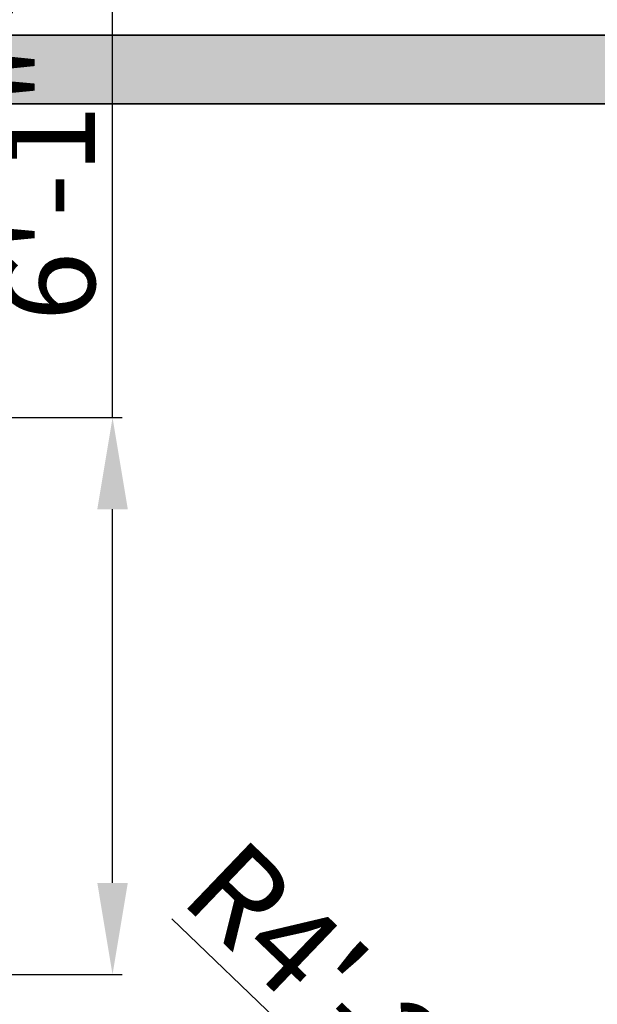
# Model space of a CAD drawing. Units: inches. Extents: x 2083 to 3317, y 1141 to 2115.
# Tile 100 of 256: x 2339 to 2415, y 1894 to 2023. Entities that reach past the tile are written whole.
import ezdxf

# ---------------------------------------------------------------- set-up
doc = ezdxf.new("R2010")
doc.units = ezdxf.units.IN
doc.layers.add('A-ANNO-DIMS', color=2, linetype='Continuous', lineweight=18)
doc.layers.add('A-WALL', color=7, linetype='Continuous', lineweight=35)
doc.layers.add('A-WALL-PATT', color=251, linetype='Continuous', lineweight=13, true_color=0x636466)
doc.styles.get("Standard").update_dxf_attribs({"font": 'arial.ttf'})
doc.dimstyles.new('ISO-25', dxfattribs={"dimtxt": 12, "dimasz": 12, "dimexe": 1.25, "dimexo": 0.625, "dimtad": 1, "dimlunit": 3, "dimtxsty": 'Standard', "dimcen": 2.5, "dimadec": 0, "dimazin": 0, "dimtfac": 1, "dimtmove": 0, "dimatfit": 3, "dimfxl": 1, "dimarcsym": 0})

# ---------------------------------------------------------------- blocks, each defined once
blk = doc.blocks.new('*D21')
at = {"layer": 'A-ANNO-DIMS', "color": 0, "lineweight": -2, "transparency": 16777216}
for p, q in [((2351.18, 1970.69), (2351.18, 2057.15)), ((2337.85, 1970.69), (2352.43, 1970.69)), ((2351.18, 1909.74), (2351.18, 1958.69)), ((2337.85, 1897.74), (2352.43, 1897.74))]:
    blk.add_line(p, q, dxfattribs=at)
at = {"layer": 'A-ANNO-DIMS', "color": 0, "transparency": 16777216}
for points in [[(2349.18, 1958.69), (2353.18, 1958.69), (2351.18, 1970.69)], [(2349.18, 1909.74), (2353.18, 1909.74), (2351.18, 1897.74)]]:
    blk.add_solid(points, dxfattribs=at)
at = {"layer": 'Defpoints', "color": 0, "transparency": 16777216}
for p in [(2337.22, 1970.69), (2351.18, 1970.69), (2337.22, 1897.74)]:
    blk.add_point(p, dxfattribs=at)
at = {"layer": 'A-ANNO-DIMS', "color": 0, "transparency": 16777216, "insert": (2344.43, 2019.92), "char_height": 12, "attachment_point": 5, "rotation": 90}
blk.add_mtext('6\'-1" TYP.', dxfattribs=at)
blk = doc.blocks.new('*D36')
at = {"layer": 'A-ANNO-DIMS', "color": 0, "lineweight": -2, "transparency": 16777216}
for p, q in [((2235.96, 2012.39), (2235.96, 2074.36)), ((2471.46, 2012.39), (2471.46, 2074.36)), ((2247.96, 2073.11), (2459.46, 2073.11))]:
    blk.add_line(p, q, dxfattribs=at)
at = {"layer": 'A-ANNO-DIMS', "color": 0, "transparency": 16777216}
for points in [[(2247.96, 2075.11), (2247.96, 2071.11), (2235.96, 2073.11)], [(2459.46, 2075.11), (2459.46, 2071.11), (2471.46, 2073.11)]]:
    blk.add_solid(points, dxfattribs=at)
at = {"layer": 'Defpoints', "color": 0, "transparency": 16777216}
for p in [(2471.46, 2073.11), (2235.96, 2011.76), (2471.46, 2011.76)]:
    blk.add_point(p, dxfattribs=at)
at = {"layer": 'A-ANNO-DIMS', "color": 0, "transparency": 16777216, "insert": (2353.71, 2079.94), "char_height": 12, "attachment_point": 5}
blk.add_mtext('19\'-7 1/2"', dxfattribs=at)
blk = doc.blocks.new('*D68')
at = {"layer": 'A-ANNO-DIMS', "color": 0, "lineweight": -2, "transparency": 16777216}
for p, q in [((2358.93, 1905.02), (2420.01, 1846.48)), ((2465.03, 1803.34), (2428.67, 1838.18))]:
    blk.add_line(p, q, dxfattribs=at)
at = {"layer": 'A-ANNO-DIMS', "color": 0, "transparency": 16777216}
blk.add_solid([(2421.39, 1847.93), (2418.62, 1845.04), (2428.67, 1838.18)], dxfattribs=at)
at = {"layer": 'Defpoints', "color": 0, "transparency": 16777216}
for p in [(2428.67, 1838.18), (2465.03, 1803.34)]:
    blk.add_point(p, dxfattribs=at)
at = {"layer": 'A-ANNO-DIMS', "color": 0, "transparency": 16777216, "insert": (2389.86, 1884.83), "char_height": 12, "attachment_point": 5, "rotation": 316.2184}
blk.add_mtext('R4\'-2 1/2"', dxfattribs=at)

msp = doc.modelspace()

# ---------------------------------------------------------------- hatches: boundary and pattern name
at = {"layer": 'A-WALL-PATT'}
h = msp.add_hatch(color=256, dxfattribs=at)
h.dxf.hatch_style = 1
h.paths.add_polyline_path([(3126.96, 2020.761), (2748.96, 2020.761), (2604.96, 2020.761), (2226.96, 2020.761), (2226.96, 1702.761), (2466.96, 1702.761), (2466.96, 1582.761), (2418.96, 1582.761), (2418.96, 1477.761), (2226.96, 1477.761), (2226.96, 1263.261), (2544.96, 1263.261), (2544.96, 1411.761), (2604.96, 1411.761), (2685.96, 1411.761), (2685.96, 1420.761), (2604.96, 1420.761), (2604.96, 1573.761), (2604.96, 1702.761), (2604.96, 2011.761), (2748.96, 2011.761), (2748.96, 1702.761), (2862.96, 1702.761), (2862.96, 1621.761), (2871.96, 1621.761), (2871.96, 1702.761), (2883.96, 1702.761), (2883.96, 1706.939, -0.0264593), (2883.96, 1711.761), (2757.96, 1711.761), (2757.96, 1807.761), (2787.96, 1807.761), (2787.96, 1812.261), (2757.96, 1812.261), (2757.96, 2011.761), (2877.96, 2011.761), (2877.96, 1812.261), (2847.96, 1812.261), (2847.96, 1807.761), (2889.836, 1807.761), (2889.836, 1812.261), (2882.46, 1812.261), (2882.46, 2011.761), (3117.96, 2011.761), (3117.96, 1812.261), (2937.836, 1812.261), (2937.836, 1807.761), (2995.71, 1807.761), (2995.71, 1796.118), (3000.21, 1796.118), (3000.21, 1807.761), (3117.96, 1807.761), (3117.96, 1711.761), (3000.21, 1711.761), (3000.21, 1760.118), (2998.573, 1760.118, -0.020711), (2995.71, 1760.118), (2995.71, 1711.761), (2931.96, 1711.761), (2931.96, 1702.761), (3126.96, 1702.761)])
h.paths.add_polyline_path([(2471.46, 2011.761), (2471.46, 1810.011), (2462.717, 1810.011), (2462.717, 1805.511), (2505.96, 1805.511), (2505.96, 1810.011), (2475.96, 1810.011), (2475.96, 2011.761), (2595.96, 2011.761), (2595.96, 1810.011), (2565.96, 1810.011), (2565.96, 1805.511), (2595.96, 1805.511), (2595.96, 1711.761), (2235.96, 1711.761), (2235.96, 1805.511), (2353.71, 1805.511), (2353.71, 1796.054), (2358.21, 1796.054), (2358.21, 1805.511), (2414.717, 1805.511), (2414.717, 1810.011), (2235.96, 1810.011), (2235.96, 2011.761)], flags=16)
h.paths.add_polyline_path([(2270.205, 1994.61), (2270.205, 1970.61), (2246.205, 1970.61), (2246.205, 1994.61)], flags=0)
edge = h.paths.add_edge_path(flags=0)
edge.add_ellipse((2332.027, 1899.798), major_axis=(-3.043, 3.043), ratio=0.1682525, start_angle=-161.33217, end_angle=-156.30711, ccw=False)
edge.add_ellipse((2333.082, 1898.744), major_axis=(-1.055, 1.055), ratio=0.4535321, start_angle=-123.37102, end_angle=-94.15911)
edge = h.paths.add_edge_path(flags=0)
edge.add_ellipse((2332.027, 1968.876), major_axis=(3.043, 3.043), ratio=0.1682525, start_angle=18.66783, end_angle=23.69289)
edge.add_spline(control_points=[(2332.926, 1970.691), (2332.227, 1970.336), (2330.894, 1969.659), (2328.413, 1970.932), (2327.204, 1967.749), (2324.71, 1969.956), (2322.533, 1967.012), (2320.013, 1971.296), (2317.68, 1968.158), (2316.041, 1967.102), (2315.427, 1966.81)], knot_values=[0, 0, 0, 0, 2.2670587, 4.3245589, 6.6855835, 8.8786411, 11.121502, 14.300359, 17.7552837, 19.732645, 19.732645, 19.732645, 19.732645], degree=3, periodic=0)
edge.add_ellipse((2332.027, 1968.876), major_axis=(3.043, 3.043), ratio=0.1682525, start_angle=18.66783, end_angle=23.69289, ccw=False)
edge.add_ellipse((2333.082, 1969.931), major_axis=(1.055, 1.055), ratio=0.4535321, start_angle=56.62898, end_angle=85.84089, ccw=False)
edge = h.paths.add_edge_path(flags=0)
edge.add_spline(control_points=[(2296.428, 1967.988), (2293.628, 1965.336), (2287.704, 1959.727), (2299.744, 1949.996), (2294.533, 1935.669), (2290.573, 1920.604), (2293.394, 1909.974), (2296.185, 1904.967)], knot_values=[0.0991853, 0.0991853, 0.0991853, 0.0991853, 0.3453009, 0.6198217, 0.9826526, 1.3860932, 1.8105546, 1.8105546, 1.8105546, 1.8105546], degree=3, periodic=0)
edge.add_spline(control_points=[(2296.185, 1904.967), (2297.384, 1902.619), (2298.001, 1901.949), (2298.553, 1901.468)], knot_values=[0.0062457, 0.0062457, 0.0062457, 0.0062457, 0.0554759, 0.0554759, 0.0554759, 0.0554759], degree=3, periodic=0)
edge.add_spline(control_points=[(2298.553, 1901.468), (2297.259, 1900.923), (2295.225, 1900.232), (2293.06, 1900.614), (2292.101, 1900.788), (2292.09, 1900.791)], knot_values=[0.3128349, 0.3128349, 0.3128349, 0.3128349, 0.4017797, 0.4749867, 0.4759027, 0.4759027, 0.4759027, 0.4759027], degree=3, periodic=0)
edge.add_arc((2292.794, 1904.664), 3.937, 215.4209, 259.69818, ccw=False)
edge.add_spline(control_points=[(2289.585, 1902.382), (2289.477, 1902.535), (2289.368, 1902.688), (2289.261, 1902.841)], knot_values=[0.1028719, 0.1028719, 0.1028719, 0.1028719, 0.1168958, 0.1168958, 0.1168958, 0.1168958], degree=3, periodic=0)
edge.add_spline(control_points=[(2289.261, 1902.841), (2288.687, 1902.55), (2287.64, 1902.02), (2285.881, 1901.874), (2283.853, 1901.504), (2281.72, 1899.711), (2278.467, 1899.493), (2276.157, 1901.883), (2272.259, 1899.804), (2267.778, 1901.843), (2262.244, 1900.184), (2257.415, 1901.782), (2254.318, 1900.726), (2253.178, 1900.337)], knot_values=[0, 0, 0, 0, 1.9079767, 3.4771759, 5.261074, 7.9728515, 11.6802485, 13.7179214, 16.9395917, 22.789562, 27.5025027, 33.5952153, 37.1456181, 37.1456181, 37.1456181, 37.1456181], degree=3, periodic=0)
edge.add_line((2253.178, 1900.337), (2250.244, 1902.841))
edge.add_line((2250.244, 1902.841), (2250.244, 1965.833))
edge.add_line((2250.244, 1965.833), (2253.178, 1968.337))
edge.add_spline(control_points=[(2253.178, 1968.337), (2254.318, 1967.948), (2257.415, 1966.892), (2262.244, 1968.49), (2267.778, 1966.831), (2271.527, 1968.537), (2273.876, 1967.828), (2274.207, 1967.728)], knot_values=[0, 0, 0, 0, 0.0901802, 0.2449351, 0.3646438, 0.5132331, 0.5378548, 0.5378548, 0.5378548, 0.5378548], degree=3, periodic=0)
edge.add_arc((2274.353, 1963.793), 3.937, 72.05113, 92.12795, ccw=False)
edge.add_arc((2281.297, 1985.23), 18.596, 252.05113, 288.56572)
edge.add_arc((2292.317, 1956.029), 12.646, 71.02679, 113.77822, ccw=False)
edge = h.paths.add_edge_path(flags=0)
edge.add_spline(control_points=[(2274.899, 1951.856), (2275.066, 1951.617), (2275.233, 1951.377), (2275.398, 1951.136)], knot_values=[1.4099157, 1.4099157, 1.4099157, 1.4099157, 1.4315903, 1.4315903, 1.4315903, 1.4315903], degree=3, periodic=0)
edge.add_spline(control_points=[(2275.398, 1951.136), (2275.792, 1950.562), (2276.179, 1949.984), (2276.546, 1949.397)], knot_values=[1.3582378, 1.3582378, 1.3582378, 1.3582378, 1.4099157, 1.4099157, 1.4099157, 1.4099157], degree=3, periodic=0)
edge.add_line((2276.546, 1949.397), (2277.437, 1947.862))
edge.add_spline(control_points=[(2277.437, 1947.862), (2276.304, 1945.673), (2274.64, 1942.427), (2274.632, 1938.094), (2272.799, 1930.852), (2274.356, 1943.897), (2275.948, 1947.923), (2276.546, 1949.397)], knot_values=[0.0056315, 0.0056315, 0.0056315, 0.0056315, 0.1860139, 0.2660015, 0.3570872, 0.5963902, 0.7397317, 0.7397317, 0.7397317, 0.7397317], degree=3, periodic=0)
edge.add_spline(control_points=[(2276.546, 1949.397), (2276.179, 1949.984), (2275.792, 1950.562), (2275.398, 1951.136)], knot_values=[1.3582378, 1.3582378, 1.3582378, 1.3582378, 1.4099157, 1.4099157, 1.4099157, 1.4099157], degree=3, periodic=0)
edge.add_spline(control_points=[(2275.398, 1951.136), (2274.943, 1950.08), (2274.208, 1948.025), (2273.935, 1944.851), (2272.469, 1937.627), (2273.466, 1945.696), (2274.701, 1951.059), (2274.899, 1951.856)], knot_values=[0.1043639, 0.1043639, 0.1043639, 0.1043639, 0.1896363, 0.2696239, 0.3607096, 0.6000126, 0.6446217, 0.6446217, 0.6446217, 0.6446217], degree=3, periodic=0)
h.paths.add_polyline_path([(2269.168, 1963.128, -0.3575267), (2268.171, 1960.976, -0.0925607), (2268.171, 1939.436, -0.3575267), (2269.168, 1937.285, -0.3575267), (2267.016, 1938.282, -0.1647847), (2254.686, 1938.282, -0.3575267), (2252.534, 1937.285, -0.3575267), (2253.531, 1939.436, -0.0925607), (2253.531, 1960.976, -0.3575267), (2252.534, 1963.128, -0.3575267), (2254.686, 1962.131, -0.1647847), (2267.016, 1962.131, -0.3575267)], flags=0)
h.paths.add_polyline_path([(2248.874, 1967.802), (2248.874, 1957.028), (2249.458, 1957.028), (2249.458, 1911.647), (2248.874, 1911.647), (2248.874, 1900.873), (2246.512, 1900.873, 0.1973271), (2244.15, 1902.457), (2244.15, 1966.218, 0.1973271), (2246.512, 1967.802)], flags=0)
h.paths.add_polyline_path([(2269.168, 1931.389, -0.3575267), (2268.171, 1929.238, -0.0925607), (2268.171, 1907.698, -0.3575267), (2269.168, 1905.547, -0.3575267), (2267.016, 1906.544, -0.1647847), (2254.686, 1906.544, -0.3575267), (2252.534, 1905.547, -0.3575267), (2253.531, 1907.698, -0.0925607), (2253.531, 1929.238, -0.3575267), (2252.534, 1931.389, -0.3575267), (2254.686, 1930.392, -0.1647847), (2267.016, 1930.392, -0.3575267)], flags=0)
edge = h.paths.add_edge_path(flags=0)
edge.add_spline(control_points=[(2276.197, 1906.724), (2276.168, 1909.029), (2276.114, 1913.372), (2270.598, 1924.925), (2273.905, 1919.013), (2275.922, 1916.262), (2275.475, 1912.402), (2277.258, 1910.381), (2276.696, 1908.225), (2276.646, 1906.813), (2276.618, 1906.008)], knot_values=[0, 0, 0, 0, 8.6102597, 16.2212739, 18.8430575, 23.8048978, 27.4408283, 29.3561016, 31.2034776, 33.6506866, 33.6506866, 33.6506866, 33.6506866], degree=3, periodic=0)
edge.add_spline(control_points=[(2276.618, 1906.008), (2276.623, 1905.624), (2276.498, 1904.629), (2275.442, 1903.855), (2274.937, 1903.08), (2274.859, 1902.841)], knot_values=[0.1564884, 0.1564884, 0.1564884, 0.1564884, 0.1843975, 0.2313765, 0.2505985, 0.2505985, 0.2505985, 0.2505985], degree=3, periodic=0)
edge.add_line((2274.859, 1902.841), (2276.506, 1902.841))
edge.add_spline(control_points=[(2276.506, 1902.841), (2276.788, 1903.085), (2277.665, 1904.125), (2278.25, 1904.341), (2277.654, 1908.527), (2278.156, 1906.228), (2278.1, 1905.286), (2278.847, 1904.069), (2277.857, 1903.415), (2277.874, 1902.991), (2277.904, 1902.841)], knot_values=[0.0595743, 0.0595743, 0.0595743, 0.0595743, 0.0807529, 0.1037415, 0.1697201, 0.1760361, 0.2071372, 0.2404744, 0.2623409, 0.2736605, 0.2736605, 0.2736605, 0.2736605], degree=3, periodic=0)
edge.add_line((2277.904, 1902.841), (2280.03, 1902.841))
edge.add_spline(control_points=[(2280.03, 1902.841), (2279.888, 1903.088), (2279.499, 1903.982), (2280.152, 1905.939), (2278.104, 1909.658), (2279.762, 1907.185), (2280.328, 1904.875), (2280.485, 1903.49), (2281.463, 1903.249), (2281.758, 1902.936), (2281.834, 1902.841)], knot_values=[0.013856, 0.013856, 0.013856, 0.013856, 0.0348738, 0.0888667, 0.1078792, 0.1267378, 0.158714, 0.1937575, 0.2174868, 0.2267221, 0.2267221, 0.2267221, 0.2267221], degree=3, periodic=0)
edge.add_spline(control_points=[(2281.834, 1902.841), (2281.788, 1902.827), (2281.647, 1902.783), (2281.396, 1902.859), (2281.088, 1902.985), (2280.721, 1903.061), (2280.333, 1903.026), (2280.125, 1902.899), (2280.03, 1902.841)], knot_values=[0, 0, 0, 0, 0.1441304, 0.435517, 0.7492759, 1.1530457, 1.5483707, 1.878348, 1.878348, 1.878348, 1.878348], degree=3, periodic=0)
edge.add_line((2280.03, 1902.841), (2277.904, 1902.841))
edge.add_spline(control_points=[(2277.904, 1902.841), (2277.893, 1902.796), (2277.865, 1902.68), (2277.607, 1902.687), (2277.274, 1902.801), (2276.838, 1902.62), (2276.584, 1902.789), (2276.506, 1902.841)], knot_values=[0, 0, 0, 0, 0.1271885, 0.3261988, 0.6280094, 1.2435704, 1.5153306, 1.5153306, 1.5153306, 1.5153306], degree=3, periodic=0)
edge.add_line((2276.506, 1902.841), (2274.859, 1902.841))
edge.add_spline(control_points=[(2274.859, 1902.841), (2274.814, 1902.899), (2274.725, 1903.013), (2274.493, 1903.119), (2274.244, 1902.961), (2273.937, 1903.185), (2273.614, 1902.983), (2273.408, 1902.883), (2273.322, 1902.841)], knot_values=[0, 0, 0, 0, 0.2184302, 0.4369566, 0.6879766, 0.9903786, 1.3983955, 1.6918498, 1.6918498, 1.6918498, 1.6918498], degree=3, periodic=0)
edge.add_spline(control_points=[(2273.322, 1902.841), (2273.617, 1903.446), (2274.274, 1904.538), (2276.027, 1904.574), (2276.207, 1906.584), (2276.197, 1906.724)], knot_values=[0.0122268, 0.0122268, 0.0122268, 0.0122268, 0.0594721, 0.1062177, 0.134458, 0.134458, 0.134458, 0.134458], degree=3, periodic=0)
h.paths.add_polyline_path([(2270.776, 1897.79), (2270.776, 1873.79), (2246.776, 1873.79), (2246.776, 1897.79)], flags=0)
h.paths.add_polyline_path([(2353.71, 1760.005), (2353.71, 1760.054), (2358.21, 1760.054, -0.033729)], flags=0)
h.paths.add_polyline_path([(2321.819, 1737.529), (2341.995, 1737.529, -0.4142136), (2343.203, 1736.321), (2343.203, 1721.021, -0.4142136), (2341.995, 1719.813), (2321.819, 1719.813, -0.4142136), (2320.611, 1721.021), (2320.611, 1736.321, -0.4142136)], flags=0)
h.paths.add_polyline_path([(2324.235, 1736.321), (2339.579, 1736.321, -0.4142136), (2341.995, 1733.905), (2341.995, 1725.45, -0.4142136), (2339.579, 1723.034), (2333.681, 1723.034), (2333.845, 1722.045, -0.8706461), (2335.425, 1721.826, -0.767327), (2333.923, 1721.423), (2331.291, 1721.423, -0.767327), (2329.788, 1721.826, -0.8706461), (2331.368, 1722.045), (2331.533, 1723.034), (2324.235, 1723.034, -0.4142136), (2321.819, 1725.45), (2321.819, 1733.905, -0.4142136)], flags=0)
h.paths.add_polyline_path([(2570.484, 1928.615), (2589.684, 1928.615), (2590.169, 1928.615), (2590.169, 1904.993), (2570.484, 1904.993)], flags=0)
h.paths.add_polyline_path([(2574.447, 1927.264, -1), (2572.829, 1927.264, -1)], flags=0)
h.paths.add_polyline_path([(2573.09, 1926.941), (2573.925, 1927.776), (2574.148, 1927.553), (2573.313, 1926.718)], flags=0)
h.paths.add_polyline_path([(2578.779, 1919.73, -1), (2571.592, 1919.73, -1)], flags=0)
h.paths.add_polyline_path([(2578.385, 1919.73, -1), (2571.985, 1919.73, -1)], flags=0)
h.paths.add_polyline_path([(2331.596, 1729.476, -1), (2333.618, 1729.476, -1)], flags=0)
h.paths.add_polyline_path([(2578.034, 1927.264, -1), (2576.416, 1927.264, -1)], flags=0)
h.paths.add_polyline_path([(2576.689, 1927.531), (2576.912, 1927.754), (2577.747, 1926.919), (2577.524, 1926.696)], flags=0)
h.paths.add_polyline_path([(2578.139, 1909.86, -1), (2572.232, 1909.86, -1)], flags=0)
h.paths.add_polyline_path([(2577.745, 1909.86, -1), (2572.625, 1909.86, -1)], flags=0)
h.paths.add_polyline_path([(2583.798, 1927.264, -1), (2582.179, 1927.264, -1)], flags=0)
h.paths.add_polyline_path([(2582.719, 1927.754), (2583.554, 1926.919), (2583.331, 1926.696), (2582.496, 1927.531)], flags=0)
h.paths.add_polyline_path([(2582.496, 1927.531), (2582.719, 1927.754), (2583.554, 1926.919), (2583.331, 1926.696)], flags=0)
h.paths.add_polyline_path([(2587.739, 1920.53, -1), (2581.832, 1920.53, -1)], flags=0)
h.paths.add_polyline_path([(2587.345, 1920.53, -1), (2582.225, 1920.53, -1)], flags=0)
h.paths.add_polyline_path([(2587.385, 1927.264, -1), (2585.766, 1927.264, -1)], flags=0)
h.paths.add_polyline_path([(2586.082, 1926.98), (2586.917, 1927.815), (2587.14, 1927.593), (2586.305, 1926.758)], flags=0)
h.paths.add_polyline_path([(2588.379, 1910.66, -1), (2581.192, 1910.66, -1)], flags=0)
h.paths.add_polyline_path([(2587.985, 1910.66, -1), (2581.585, 1910.66, -1)], flags=0)
h.paths.add_polyline_path([(2417.168, 1729.478), (2437.344, 1729.478, -0.4142136), (2438.552, 1728.27), (2438.552, 1712.969, -0.4142136), (2437.344, 1711.761), (2417.168, 1711.761, -0.4142136), (2415.96, 1712.969), (2415.96, 1728.27, -0.4142136)], flags=0)
h.paths.add_polyline_path([(2419.584, 1728.27), (2434.928, 1728.27, -0.4142136), (2437.344, 1725.854), (2437.344, 1717.398, -0.4142136), (2434.928, 1714.983), (2429.029, 1714.983), (2429.194, 1713.994, -0.8706461), (2430.774, 1713.775, -0.767327), (2429.271, 1713.372), (2426.64, 1713.372, -0.767327), (2425.137, 1713.775, -0.8706461), (2426.717, 1713.994), (2426.882, 1714.983), (2419.584, 1714.983, -0.4142136), (2417.168, 1717.398), (2417.168, 1725.854, -0.4142136)], flags=0)
h.paths.add_polyline_path([(2419.584, 1728.27), (2434.928, 1728.27, -0.4142136), (2437.344, 1725.854), (2437.344, 1717.398, -0.4142136), (2434.928, 1714.983), (2429.029, 1714.983), (2428.358, 1719.009), (2427.553, 1719.009), (2426.882, 1714.983), (2419.584, 1714.983, -0.4142136), (2417.168, 1717.398), (2417.168, 1725.854, -0.4142136)], flags=0)
h.paths.add_polyline_path([(2426.944, 1721.425, -1), (2428.967, 1721.425, -1)], flags=0)
h.paths.add_polyline_path([(2475.96, 1702.761), (2595.96, 1702.761), (2595.96, 1582.761), (2475.96, 1582.761)], flags=16)
h.paths.add_polyline_path([(2427.96, 1573.761), (2595.96, 1573.761), (2595.96, 1468.761), (2595.96, 1420.761), (2384.46, 1420.761), (2384.46, 1468.761), (2427.96, 1468.761)], flags=16)
h.paths.add_polyline_path([(2379.96, 1468.761), (2379.96, 1420.761), (2235.96, 1420.761), (2235.96, 1468.761)], flags=16)
h.paths.add_polyline_path([(2317.816, 1466.696), (2337.992, 1466.696, -0.4142136), (2339.2, 1465.488), (2339.2, 1450.187, -0.4142136), (2337.992, 1448.979), (2317.816, 1448.979, -0.4142136), (2316.608, 1450.187), (2316.608, 1465.488, -0.4142136)], flags=0)
h.paths.add_polyline_path([(2320.232, 1465.488), (2335.576, 1465.488, -0.4142136), (2337.992, 1463.072), (2337.992, 1454.616, -0.4142136), (2335.576, 1452.2), (2329.677, 1452.2), (2329.842, 1451.212, -0.8706461), (2331.422, 1450.992, -0.767327), (2329.92, 1450.59), (2327.288, 1450.59, -0.767327), (2325.785, 1450.992, -0.8706461), (2327.365, 1451.212), (2327.53, 1452.2), (2320.232, 1452.2, -0.4142136), (2317.816, 1454.616), (2317.816, 1463.072, -0.4142136)], flags=0)
h.paths.add_polyline_path([(2320.232, 1465.488), (2335.576, 1465.488, -0.4142136), (2337.992, 1463.072), (2337.992, 1454.616, -0.4142136), (2335.576, 1452.2), (2329.677, 1452.2), (2329.006, 1456.227), (2328.201, 1456.227), (2327.53, 1452.2), (2320.232, 1452.2, -0.4142136), (2317.816, 1454.616), (2317.816, 1463.072, -0.4142136)], flags=0)
h.paths.add_polyline_path([(2327.593, 1458.643, -1), (2329.615, 1458.643, -1)], flags=0)
h.paths.add_polyline_path([(2244.412, 1433.34), (2241.921, 1433.34, -0.4142136), (2240.018, 1435.244), (2240.018, 1440.953, -0.4142105), (2241.921, 1442.856), (2244.412, 1442.856, -1.9764724)], flags=0)
h.paths.add_polyline_path([(2245.357, 1434.398, -0.4142136), (2245.357, 1441.799, -2.1440985)], flags=0)
h.paths.add_polyline_path([(2535.96, 1416.261), (2535.96, 1272.261), (2235.96, 1272.261), (2235.96, 1416.261)], flags=16)
h.paths.add_polyline_path([(2260.12, 1384.293), (2260.12, 1362.039), (2237.865, 1362.039), (2237.865, 1384.293)], flags=0)
edge = h.paths.add_edge_path(flags=0)
edge.add_line((2318.252, 1362.093), (2318.146, 1362.001))
edge.add_ellipse((2317.445, 1360.431), major_axis=(2.822, 2.822), ratio=0.1682525, start_angle=18.66783, end_angle=20.94813, ccw=False)
edge.add_ellipse((2318.423, 1361.409), major_axis=(0.978, 0.978), ratio=0.4535321, start_angle=56.62898, end_angle=70.2262, ccw=False)
edge = h.paths.add_edge_path(flags=0)
edge.add_line((2319.107, 1295.571), (2319.015, 1295.677))
edge.add_ellipse((2317.445, 1296.378), major_axis=(-2.822, 2.822), ratio=0.1682525, start_angle=-161.33217, end_angle=-159.05187, ccw=False)
edge.add_ellipse((2318.423, 1295.4), major_axis=(-0.978, 0.978), ratio=0.4535321, start_angle=-123.37102, end_angle=-109.7738)
edge = h.paths.add_edge_path(flags=0)
edge.add_spline(control_points=[(2284.21, 1301.17), (2284.581, 1300.445), (2284.891, 1299.892), (2285.16, 1299.461)], knot_values=[0.0390658, 0.0390658, 0.0390658, 0.0390658, 0.0554759, 0.0554759, 0.0554759, 0.0554759], degree=3, periodic=0)
edge.add_line((2285.16, 1299.461), (2284.21, 1301.17))
edge = h.paths.add_edge_path(flags=0)
edge.add_line((2280.412, 1297.298), (2283.37, 1297.036))
edge.add_line((2283.37, 1297.036), (2286.406, 1297.926))
edge.add_spline(control_points=[(2286.406, 1297.926), (2285.305, 1297.463), (2284.345, 1297.129), (2283.37, 1297.036)], knot_values=[0.3943688, 0.3943688, 0.3943688, 0.3943688, 0.4759027, 0.4759027, 0.4759027, 0.4759027], degree=3, periodic=0)
edge.add_spline(control_points=[(2283.37, 1297.036), (2283.281, 1297.028), (2282.316, 1296.957), (2281.313, 1297.134), (2280.423, 1297.296), (2280.412, 1297.298)], knot_values=[0.3128349, 0.3128349, 0.3128349, 0.3128349, 0.3202458, 0.3934528, 0.3943688, 0.3943688, 0.3943688, 0.3943688], degree=3, periodic=0)
edge = h.paths.add_edge_path(flags=0)
edge.add_line((2284.436, 1359.607), (2280.446, 1355.328))
edge.add_line((2280.446, 1355.328), (2279.58, 1351.018))
edge.add_line((2279.58, 1351.018), (2282.413, 1346.58))
edge.add_spline(control_points=[(2282.413, 1346.58), (2283.153, 1345.589), (2284.253, 1344.029), (2284.801, 1342.387), (2284.935, 1341.806)], knot_values=[1.2400982, 1.2400982, 1.2400982, 1.2400982, 1.3328922, 1.3827123, 1.3827123, 1.3827123, 1.3827123], degree=3, periodic=0)
edge.add_spline(control_points=[(2284.935, 1341.806), (2285.319, 1340.141), (2285.233, 1338.409), (2284.91, 1336.654)], knot_values=[1.0974841, 1.0974841, 1.0974841, 1.0974841, 1.2400982, 1.2400982, 1.2400982, 1.2400982], degree=3, periodic=0)
edge.add_spline(control_points=[(2284.91, 1336.654), (2284.587, 1334.899), (2284.027, 1333.12), (2283.463, 1331.361)], knot_values=[0.9548699, 0.9548699, 0.9548699, 0.9548699, 1.0974841, 1.0974841, 1.0974841, 1.0974841], degree=3, periodic=0)
edge.add_line((2283.463, 1331.361), (2281.89, 1326.153))
edge.add_line((2281.89, 1326.153), (2280.756, 1321.056))
edge.add_line((2280.756, 1321.056), (2280.299, 1316.002))
edge.add_line((2280.299, 1316.002), (2280.716, 1310.95))
edge.add_line((2280.716, 1310.95), (2282.028, 1305.972))
edge.add_line((2282.028, 1305.972), (2284.21, 1301.17))
edge.add_spline(control_points=[(2284.21, 1301.17), (2283.341, 1302.73), (2282.612, 1304.336), (2282.028, 1305.972)], knot_values=[0.0991853, 0.0991853, 0.0991853, 0.0991853, 0.2417994, 0.2417994, 0.2417994, 0.2417994], degree=3, periodic=0)
edge.add_spline(control_points=[(2282.028, 1305.972), (2281.444, 1307.608), (2281.005, 1309.273), (2280.716, 1310.95)], knot_values=[0.2417994, 0.2417994, 0.2417994, 0.2417994, 0.3844135, 0.3844135, 0.3844135, 0.3844135], degree=3, periodic=0)
edge.add_spline(control_points=[(2280.716, 1310.95), (2280.433, 1312.588), (2280.289, 1314.277), (2280.299, 1315.962), (2280.299, 1316.002)], knot_values=[0.3844135, 0.3844135, 0.3844135, 0.3844135, 0.5236467, 0.5270276, 0.5270276, 0.5270276, 0.5270276], degree=3, periodic=0)
edge.add_spline(control_points=[(2280.299, 1316.002), (2280.312, 1317.687), (2280.478, 1319.368), (2280.756, 1321.056)], knot_values=[0.5270276, 0.5270276, 0.5270276, 0.5270276, 0.6696417, 0.6696417, 0.6696417, 0.6696417], degree=3, periodic=0)
edge.add_spline(control_points=[(2280.756, 1321.056), (2281.035, 1322.744), (2281.426, 1324.44), (2281.89, 1326.153)], knot_values=[0.6696417, 0.6696417, 0.6696417, 0.6696417, 0.8122558, 0.8122558, 0.8122558, 0.8122558], degree=3, periodic=0)
edge.add_spline(control_points=[(2281.89, 1326.153), (2282.264, 1327.533), (2282.788, 1329.262), (2283.353, 1331.018), (2283.463, 1331.361)], knot_values=[0.8122558, 0.8122558, 0.8122558, 0.8122558, 0.9270873, 0.9548699, 0.9548699, 0.9548699, 0.9548699], degree=3, periodic=0)
edge.add_line((2283.463, 1331.361), (2284.91, 1336.654))
edge.add_line((2284.91, 1336.654), (2284.935, 1341.806))
edge.add_line((2284.935, 1341.806), (2282.413, 1346.58))
edge.add_spline(control_points=[(2282.413, 1346.58), (2281.275, 1348.104), (2280.078, 1349.57), (2279.58, 1351.018)], knot_values=[1.3827123, 1.3827123, 1.3827123, 1.3827123, 1.5253264, 1.5253264, 1.5253264, 1.5253264], degree=3, periodic=0)
edge.add_spline(control_points=[(2279.58, 1351.018), (2279.443, 1351.415), (2279.136, 1352.857), (2279.735, 1354.29), (2280.446, 1355.328)], knot_values=[1.5253264, 1.5253264, 1.5253264, 1.5253264, 1.564439, 1.6679405, 1.6679405, 1.6679405, 1.6679405], degree=3, periodic=0)
edge.add_spline(control_points=[(2280.446, 1355.328), (2281.426, 1356.758), (2282.931, 1358.183), (2284.436, 1359.607)], knot_values=[1.6679405, 1.6679405, 1.6679405, 1.6679405, 1.8105546, 1.8105546, 1.8105546, 1.8105546], degree=3, periodic=0)
edge.add_arc((2280.623, 1348.518), 11.726, 71.02679, 113.77822)
edge.add_arc((2270.405, 1375.595), 17.244, 252.05113, 288.56572, ccw=False)
edge.add_arc((2263.966, 1355.718), 3.651, 72.05113, 92.12795)
edge.add_arc((2263.966, 1355.718), 3.651, 92.12795, 177.98513)
edge.add_spline(control_points=[(2260.318, 1355.846), (2260.26, 1354.221), (2260.551, 1350.187), (2262.999, 1346.766), (2264.473, 1344.649)], knot_values=[1.4315903, 1.4315903, 1.4315903, 1.4315903, 1.5641438, 1.7706953, 1.7706953, 1.7706953, 1.7706953], degree=3, periodic=0)
edge.add_line((2264.473, 1344.649), (2264.936, 1343.983))
edge.add_spline(control_points=[(2263.801, 1340.248), (2263.843, 1340.514), (2264.067, 1341.756), (2264.513, 1343.002), (2264.935, 1343.981)], knot_values=[0.5365702, 0.5365702, 0.5365702, 0.5365702, 0.5593494, 0.6446217, 0.6446217, 0.6446217, 0.6446217], degree=3, periodic=0)
edge.add_spline(control_points=[(2264.935, 1343.981), (2265.118, 1343.715), (2265.299, 1343.448), (2265.477, 1343.179)], knot_values=[1.3840767, 1.3840767, 1.3840767, 1.3840767, 1.4099157, 1.4099157, 1.4099157, 1.4099157], degree=3, periodic=0)
edge.add_spline(control_points=[(2265.477, 1343.179), (2265.655, 1342.911), (2265.829, 1342.641), (2265.999, 1342.369)], knot_values=[1.3582378, 1.3582378, 1.3582378, 1.3582378, 1.3840767, 1.3840767, 1.3840767, 1.3840767], degree=3, periodic=0)
edge.add_line((2265.999, 1342.369), (2266.826, 1340.946))
edge.add_spline(control_points=[(2266.826, 1340.946), (2268.894, 1337.09), (2271.398, 1325.843), (2270.516, 1310.569), (2275.919, 1301.861), (2277.79, 1299.199)], knot_values=[0.1168958, 0.1168958, 0.1168958, 0.1168958, 0.4729873, 1.0509689, 1.3137934, 1.3137934, 1.3137934, 1.3137934], degree=3, periodic=0)
edge.add_spline(control_points=[(2277.79, 1299.199), (2277.839, 1299.128), (2277.889, 1299.057), (2277.94, 1298.987)], knot_values=[0.1098839, 0.1098839, 0.1098839, 0.1098839, 0.1168958, 0.1168958, 0.1168958, 0.1168958], degree=3, periodic=0)
edge.add_line((2277.94, 1298.987), (2277.789, 1299.199))
edge.add_spline(control_points=[(2277.789, 1299.199), (2277.257, 1298.929), (2276.286, 1298.438), (2275.039, 1298.334), (2274.383, 1298.239), (2274.215, 1298.209)], knot_values=[33.1218702, 33.1218702, 33.1218702, 33.1218702, 35.0290557, 36.5982549, 37.1448269, 37.1448269, 37.1448269, 37.1448269], degree=3, periodic=0)
edge.add_line((2274.215, 1298.209), (2273.073, 1297.893))
edge.add_spline(control_points=[(2273.073, 1297.893), (2272.323, 1297.58), (2271.039, 1296.511), (2269.248, 1296.226), (2268.423, 1296.375)], knot_values=[26.5325843, 26.5325843, 26.5325843, 26.5325843, 29.198919, 31.8391012, 31.8391012, 31.8391012, 31.8391012], degree=3, periodic=0)
edge.add_line((2268.423, 1296.375), (2263.879, 1297.458))
edge.add_spline(control_points=[(2263.879, 1297.458), (2263.556, 1297.359), (2261.86, 1296.839), (2260.239, 1297.282), (2258.933, 1297.516)], knot_values=[15.9195506, 15.9195506, 15.9195506, 15.9195506, 16.9395917, 21.2260675, 21.2260675, 21.2260675, 21.2260675], degree=3, periodic=0)
edge.add_line((2258.933, 1297.516), (2254.055, 1297.329))
edge.add_spline(control_points=[(2254.055, 1297.329), (2253.756, 1297.296), (2252.114, 1297.165), (2250.462, 1297.544), (2249.13, 1297.668)], knot_values=[5.3065169, 5.3065169, 5.3065169, 5.3065169, 6.2764352, 10.6130337, 10.6130337, 10.6130337, 10.6130337], degree=3, periodic=0)
edge.add_line((2249.13, 1297.668), (2244.332, 1296.878))
edge.add_line((2244.332, 1296.878), (2241.611, 1299.199))
edge.add_line((2241.611, 1299.199), (2241.611, 1357.609))
edge.add_line((2241.611, 1357.609), (2244.332, 1359.931))
edge.add_line((2244.332, 1359.931), (2252.729, 1359.543))
edge.add_spline(control_points=[(2252.729, 1359.543), (2252.871, 1359.546), (2253.306, 1359.548), (2253.74, 1359.514), (2254.032, 1359.482)], knot_values=[0.233291, 0.233291, 0.233291, 0.233291, 0.2449351, 0.2689274, 0.2689274, 0.2689274, 0.2689274], degree=3, periodic=0)
edge.add_line((2254.032, 1359.482), (2259.587, 1359.416))
edge.add_spline(control_points=[(2259.587, 1359.416), (2260.677, 1359.629), (2262.073, 1359.897), (2263.524, 1359.459), (2263.83, 1359.366)], knot_values=[0.4225164, 0.4225164, 0.4225164, 0.4225164, 0.5132331, 0.5378548, 0.5378548, 0.5378548, 0.5378548], degree=3, periodic=0)
edge.add_arc((2263.966, 1355.718), 3.651, 72.05113, 92.12795, ccw=False)
edge.add_arc((2270.405, 1375.595), 17.244, 252.05113, 288.56572)
edge.add_arc((2280.623, 1348.518), 11.726, 71.02679, 113.77822, ccw=False)
h.paths.add_polyline_path([(2240.341, 1359.435), (2240.341, 1349.444), (2240.882, 1349.444), (2240.882, 1307.365), (2240.341, 1307.365), (2240.341, 1297.374), (2238.15, 1297.374, 0.1973271), (2235.96, 1298.843), (2235.96, 1357.966, 0.1973271), (2238.15, 1359.435)], flags=0)
h.paths.add_polyline_path([(2259.158, 1355.101, -0.3575267), (2258.233, 1353.106, -0.0925607), (2258.233, 1333.133, -0.3575267), (2259.158, 1331.138, -0.3575267), (2257.163, 1332.062, -0.1647847), (2245.729, 1332.062, -0.3575267), (2243.735, 1331.138, -0.3575267), (2244.659, 1333.133, -0.0925607), (2244.659, 1353.106, -0.3575267), (2243.735, 1355.101, -0.3575267), (2245.729, 1354.176, -0.1647847), (2257.163, 1354.176, -0.3575267)], flags=0)
edge = h.paths.add_edge_path(flags=0)
edge.add_line((2265.999, 1342.369), (2266.826, 1340.946))
edge.add_line((2266.826, 1340.946), (2265.308, 1337.814))
edge.add_line((2265.308, 1337.814), (2264.358, 1334.653))
edge.add_line((2264.358, 1334.653), (2264.262, 1333.8))
edge.add_spline(control_points=[(2264.262, 1333.8), (2264.208, 1333.187), (2264.162, 1332.366), (2264.007, 1331.414), (2263.969, 1331.202)], knot_values=[0.4644442, 0.4644442, 0.4644442, 0.4644442, 0.5166905, 0.5316081, 0.5316081, 0.5316081, 0.5316081], degree=3, periodic=0)
edge.add_spline(control_points=[(2263.969, 1331.202), (2263.775, 1330.119), (2263.424, 1328.791), (2263.257, 1328.531), (2263.234, 1328.515)], knot_values=[0.3726816, 0.3726816, 0.3726816, 0.3726816, 0.4488497, 0.4644442, 0.4644442, 0.4644442, 0.4644442], degree=3, periodic=0)
edge.add_spline(control_points=[(2263.234, 1328.515), (2263.096, 1328.42), (2263.131, 1329.301), (2263.275, 1330.616)], knot_values=[0.2809191, 0.2809191, 0.2809191, 0.2809191, 0.3726816, 0.3726816, 0.3726816, 0.3726816], degree=3, periodic=0)
edge.add_spline(control_points=[(2263.275, 1330.616), (2263.419, 1331.93), (2263.672, 1333.677), (2263.97, 1335.315)], knot_values=[0.1891566, 0.1891566, 0.1891566, 0.1891566, 0.2809191, 0.2809191, 0.2809191, 0.2809191], degree=3, periodic=0)
edge.add_spline(control_points=[(2263.97, 1335.315), (2264.1, 1336.032), (2264.419, 1337.622), (2264.755, 1338.864), (2264.947, 1339.491)], knot_values=[0.097394, 0.097394, 0.097394, 0.097394, 0.1375775, 0.1891566, 0.1891566, 0.1891566, 0.1891566], degree=3, periodic=0)
edge.add_spline(control_points=[(2264.947, 1339.491), (2265.29, 1340.606), (2265.644, 1341.494), (2265.999, 1342.369)], knot_values=[0.0056315, 0.0056315, 0.0056315, 0.0056315, 0.097394, 0.097394, 0.097394, 0.097394], degree=3, periodic=0)
h.paths.add_polyline_path([(2259.158, 1325.671, -0.3575267), (2258.233, 1323.676, -0.0925607), (2258.233, 1303.703, -0.3575267), (2259.158, 1301.708, -0.3575267), (2257.163, 1302.633, -0.1647847), (2245.729, 1302.633, -0.3575267), (2243.735, 1301.708, -0.3575267), (2244.659, 1303.703, -0.0925607), (2244.659, 1323.676, -0.3575267), (2243.735, 1325.671, -0.3575267), (2245.729, 1324.747, -0.1647847), (2257.163, 1324.747, -0.3575267)], flags=0)
edge = h.paths.add_edge_path(flags=0)
edge.add_spline(control_points=[(2261.709, 1317.311), (2261.679, 1317.418), (2261.762, 1317.389), (2262.491, 1316.09), (2262.962, 1315.301)], knot_values=[14.9558607, 14.9558607, 14.9558607, 14.9558607, 16.2212739, 18.6948259, 18.6948259, 18.6948259, 18.6948259], degree=3, periodic=0)
edge.add_spline(control_points=[(2262.962, 1315.301), (2262.99, 1315.254), (2263.702, 1314.067), (2264.349, 1313.127), (2264.73, 1312.164)], knot_values=[18.6948259, 18.6948259, 18.6948259, 18.6948259, 18.8430575, 22.433791, 22.433791, 22.433791, 22.433791], degree=3, periodic=0)
edge.add_spline(control_points=[(2264.73, 1312.164), (2264.876, 1311.796), (2265.177, 1310.77), (2265.143, 1309.559), (2265.248, 1308.824)], knot_values=[22.433791, 22.433791, 22.433791, 22.433791, 23.8048978, 26.1727562, 26.1727562, 26.1727562, 26.1727562], degree=3, periodic=0)
edge.add_line((2265.248, 1308.824), (2265.851, 1307.172))
edge.add_spline(control_points=[(2265.851, 1307.172), (2266.065, 1306.822), (2266.384, 1306.332), (2266.424, 1305.781), (2266.42, 1305.611)], knot_values=[28.0625624, 28.0625624, 28.0625624, 28.0625624, 29.3561016, 29.9117214, 29.9117214, 29.9117214, 29.9117214], degree=3, periodic=0)
edge.add_spline(control_points=[(2266.42, 1305.611), (2266.416, 1305.433), (2266.394, 1305.25), (2266.365, 1305.066)], knot_values=[29.9117214, 29.9117214, 29.9117214, 29.9117214, 30.4978371, 30.4978371, 30.4978371, 30.4978371], degree=3, periodic=0)
edge.add_line((2266.365, 1305.066), (2266.066, 1302.136))
edge.add_spline(control_points=[(2266.066, 1302.136), (2266.071, 1301.78), (2265.998, 1301.2), (2265.663, 1300.759), (2265.509, 1300.586)], knot_values=[0.1564884, 0.1564884, 0.1564884, 0.1564884, 0.1843975, 0.2035434, 0.2035434, 0.2035434, 0.2035434], degree=3, periodic=0)
edge.add_line((2265.509, 1300.586), (2264.435, 1299.199))
edge.add_line((2264.435, 1299.199), (2265.962, 1299.199))
edge.add_line((2265.962, 1299.199), (2267.336, 1301.175))
edge.add_line((2267.336, 1301.175), (2267.312, 1301.986))
edge.add_spline(control_points=[(2267.312, 1301.986), (2267.261, 1302.862), (2267.16, 1303.737), (2267.271, 1303.326)], knot_values=[0.1262286, 0.1262286, 0.1262286, 0.1262286, 0.1666174, 0.1666174, 0.1666174, 0.1666174], degree=3, periodic=0)
edge.add_spline(control_points=[(2267.271, 1303.326), (2267.28, 1303.294), (2267.31, 1303.175), (2267.373, 1302.884), (2267.406, 1302.683), (2267.418, 1302.601)], knot_values=[0.1666174, 0.1666174, 0.1666174, 0.1666174, 0.1697201, 0.1760361, 0.1807647, 0.1807647, 0.1807647, 0.1807647], degree=3, periodic=0)
edge.add_spline(control_points=[(2267.744, 1300.988), (2267.688, 1301.151), (2267.481, 1301.657), (2267.484, 1302.145), (2267.418, 1302.601)], knot_values=[0.1807647, 0.1807647, 0.1807647, 0.1807647, 0.1937665, 0.2201389, 0.2201389, 0.2201389, 0.2201389], degree=3, periodic=0)
edge.add_line((2267.418, 1302.601), (2267.744, 1300.988))
edge.add_spline(control_points=[(2267.744, 1300.988), (2267.832, 1300.732), (2267.932, 1300.31), (2267.555, 1299.975), (2267.429, 1299.829)], knot_values=[0.2201389, 0.2201389, 0.2201389, 0.2201389, 0.2404744, 0.2548903, 0.2548903, 0.2548903, 0.2548903], degree=3, periodic=0)
edge.add_line((2267.429, 1299.829), (2267.258, 1299.199))
edge.add_line((2267.258, 1299.199), (2269.23, 1299.199))
edge.add_spline(control_points=[(2269.23, 1299.199), (2269.099, 1299.429), (2268.843, 1300.016), (2269.012, 1300.916), (2268.947, 1301.661)], knot_values=[0.013856, 0.013856, 0.013856, 0.013856, 0.0348738, 0.0670726, 0.0670726, 0.0670726, 0.0670726], degree=3, periodic=0)
edge.add_line((2268.947, 1301.661), (2268.432, 1303.603))
edge.add_spline(control_points=[(2268.432, 1303.603), (2268.176, 1304.192), (2267.596, 1305.251), (2268.041, 1304.623), (2268.251, 1304.282)], knot_values=[0.0901547, 0.0901547, 0.0901547, 0.0901547, 0.1078792, 0.1202891, 0.1202891, 0.1202891, 0.1202891], degree=3, periodic=0)
edge.add_spline(control_points=[(2268.251, 1304.282), (2268.361, 1304.105), (2269.058, 1302.918), (2269.383, 1301.59), (2269.521, 1300.776), (2269.575, 1300.556)], knot_values=[0.1202891, 0.1202891, 0.1202891, 0.1202891, 0.1267378, 0.158714, 0.1735056, 0.1735056, 0.1735056, 0.1735056], degree=3, periodic=0)
edge.add_line((2269.575, 1300.556), (2270.686, 1299.421))
edge.add_spline(control_points=[(2270.686, 1299.421), (2270.767, 1299.357), (2270.838, 1299.281), (2270.903, 1299.199)], knot_values=[0.2181597, 0.2181597, 0.2181597, 0.2181597, 0.2267221, 0.2267221, 0.2267221, 0.2267221], degree=3, periodic=0)
edge.add_line((2270.937, 1299.193), (2270.903, 1299.199))
edge.add_spline(control_points=[(2270.903, 1299.199), (2270.86, 1299.186), (2270.73, 1299.146), (2270.496, 1299.216), (2270.272, 1299.308), (2270.121, 1299.348), (2270.063, 1299.36)], knot_values=[0.939174, 0.939174, 0.939174, 0.939174, 1.0833044, 1.3746911, 1.6884499, 1.878348, 1.878348, 1.878348, 1.878348], degree=3, periodic=0)
edge.add_line((2270.063, 1299.36), (2269.23, 1299.199))
edge.add_line((2269.23, 1299.199), (2267.258, 1299.199))
edge.add_spline(control_points=[(2267.258, 1299.199), (2267.248, 1299.157), (2267.223, 1299.05), (2266.984, 1299.057), (2266.809, 1299.116), (2266.677, 1299.109), (2266.637, 1299.105)], knot_values=[0.7576653, 0.7576653, 0.7576653, 0.7576653, 0.8848538, 1.0838641, 1.3856747, 1.5153306, 1.5153306, 1.5153306, 1.5153306], degree=3, periodic=0)
edge.add_spline(control_points=[(2266.637, 1299.105), (2266.485, 1299.089), (2266.236, 1299.017), (2266.035, 1299.151), (2265.962, 1299.199)], knot_values=[0, 0, 0, 0, 0.4859051, 0.7576653, 0.7576653, 0.7576653, 0.7576653], degree=3, periodic=0)
edge.add_line((2265.962, 1299.199), (2264.435, 1299.199))
edge.add_line((2264.435, 1299.199), (2263.858, 1299.367))
edge.add_spline(control_points=[(2263.858, 1299.367), (2263.819, 1299.371), (2263.78, 1299.386), (2263.74, 1299.402)], knot_values=[0.8459249, 0.8459249, 0.8459249, 0.8459249, 0.9786272, 0.9786272, 0.9786272, 0.9786272], degree=3, periodic=0)
edge.add_line((2263.722, 1299.396), (2263.01, 1299.199))
edge.add_spline(control_points=[(2263.01, 1299.199), (2263.246, 1299.683), (2263.506, 1300.128), (2263.873, 1300.408)], knot_values=[0.0122268, 0.0122268, 0.0122268, 0.0122268, 0.0529705, 0.0529705, 0.0529705, 0.0529705], degree=3, periodic=0)
edge.add_spline(control_points=[(2263.873, 1300.408), (2263.932, 1300.453), (2264.084, 1300.553), (2264.255, 1300.624), (2264.36, 1300.665)], knot_values=[0.0529705, 0.0529705, 0.0529705, 0.0529705, 0.0594721, 0.0690861, 0.0690861, 0.0690861, 0.0690861], degree=3, periodic=0)
edge.add_line((2264.36, 1300.665), (2265.142, 1301.078))
edge.add_line((2265.142, 1301.078), (2265.676, 1302.8))
edge.add_line((2265.676, 1302.8), (2265.541, 1305.704))
edge.add_line((2265.541, 1305.704), (2264.803, 1309.328))
edge.add_line((2264.803, 1309.328), (2263.041, 1314.092))
edge.add_spline(control_points=[(2263.041, 1314.092), (2262.384, 1315.671), (2261.796, 1316.998), (2261.709, 1317.311)], knot_values=[11.2168955, 11.2168955, 11.2168955, 11.2168955, 14.9558607, 14.9558607, 14.9558607, 14.9558607], degree=3, periodic=0)
h.paths.add_polyline_path([(2871.96, 1416.261), (2895.91, 1416.261), (2895.91, 1420.761), (2871.96, 1420.761), (2871.96, 1501.761), (2862.96, 1501.761), (2862.96, 1420.761), (2805.96, 1420.761), (2805.96, 1411.761), (2862.96, 1411.761), (2862.96, 1263.261), (3126.96, 1263.261), (3126.96, 1411.761), (3126.96, 1486.761), (2943.96, 1486.761), (2943.96, 1477.761), (2967.86, 1477.761), (2967.86, 1420.761), (2943.91, 1420.761), (2943.91, 1416.261), (3117.96, 1416.261), (3117.96, 1420.761), (2972.36, 1420.761), (2972.36, 1477.761), (3117.96, 1477.761), (3117.96, 1420.761), (3117.96, 1272.261), (2871.96, 1272.261)], flags=0)
h.paths.add_polyline_path([(2457.126, 1485.943), (2527.603, 1485.943), (2527.603, 1537.636), (2457.126, 1537.636)], flags=8)
h.paths.add_polyline_path([(2481.005, 1609.982), (2590.766, 1609.982), (2590.766, 1682.003), (2481.005, 1682.003)], flags=8)
h.paths.add_polyline_path([(2483.085, 1729.127), (2553.562, 1729.127), (2553.562, 1780.82), (2483.085, 1780.82)], flags=8)

# ---------------------------------------------------------------- linework, layer by layer
at = {"layer": 'A-WALL'}
for p, q in [((2226.96, 2020.761), (2604.96, 2020.761)), ((2235.96, 2011.761), (2471.46, 2011.761))]:
    msp.add_line(p, q, dxfattribs=at)

# ---------------------------------------------------------------- dimensions: what is measured, and where the dimension line sits
at = {"layer": 'A-ANNO-DIMS'}
dim = msp.add_linear_dim(base=(2471.46, 2073.111), p1=(2235.96, 2011.761), p2=(2471.46, 2011.761), dimstyle='ISO-25', override={"dimdec": 1, "dimlfac": 1, "dimrnd": 0, "dimzin": 1, "dimdsep": 46, "dimlunit": 4, "dimfrac": 2}, dxfattribs=at)
dim.commit()
dim.dimension.update_dxf_attribs({"geometry": '*D36', "text_midpoint": (2353.71, 2079.941)})
dim = msp.add_linear_dim(base=(2351.181, 1970.691), p1=(2337.22, 1897.744), p2=(2337.22, 1970.691), angle=90, text='<> TYP.', dimstyle='ISO-25', override={"dimdec": 1, "dimlfac": 1, "dimrnd": 0, "dimzin": 1, "dimdsep": 46, "dimlunit": 4, "dimfrac": 2}, dxfattribs=at)
dim.commit()
dim.dimension.update_dxf_attribs({"geometry": '*D21', "text_midpoint": (2344.429, 2019.922)})
dim = msp.add_radius_dim(center=(2465.03, 1803.336), mpoint=(2428.671, 1838.181), dimstyle='ISO-25', override={"dimdec": 1, "dimlfac": 1, "dimrnd": 0, "dimzin": 1, "dimdsep": 46, "dimlunit": 4, "dimfrac": 2}, dxfattribs=at)
dim.commit()
dim.dimension.update_dxf_attribs({"geometry": '*D68', "text_midpoint": (2389.863, 1884.833)})

doc.saveas('drawing.dxf')
